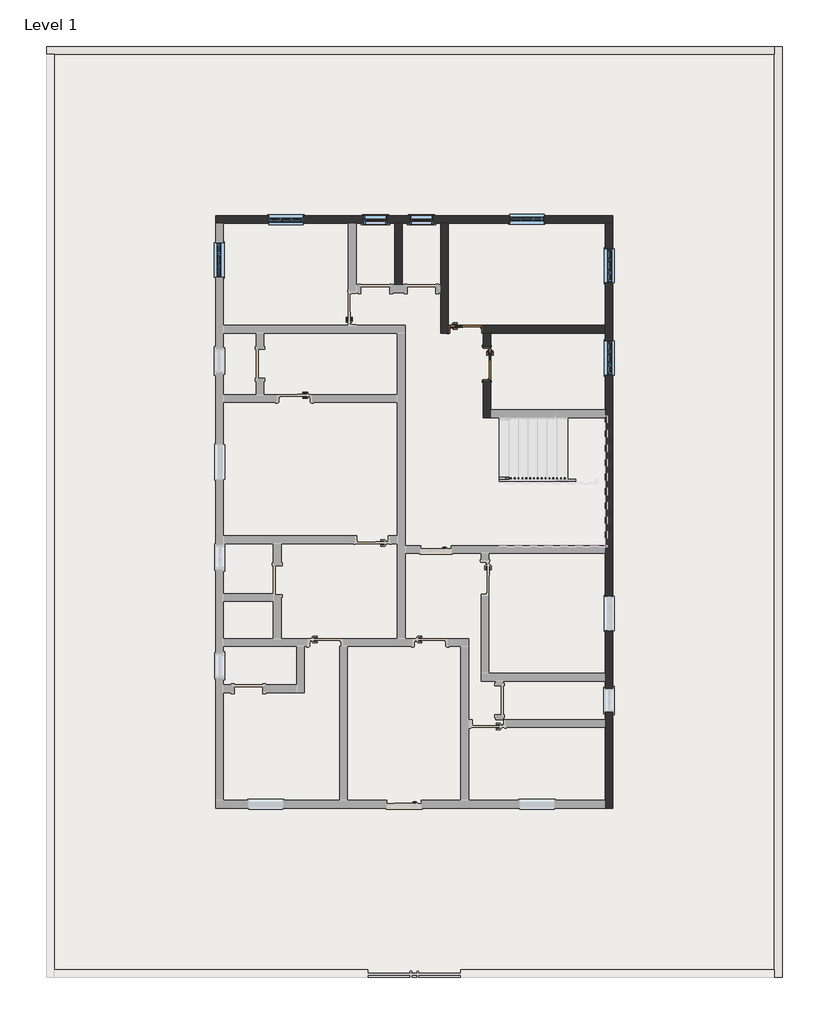
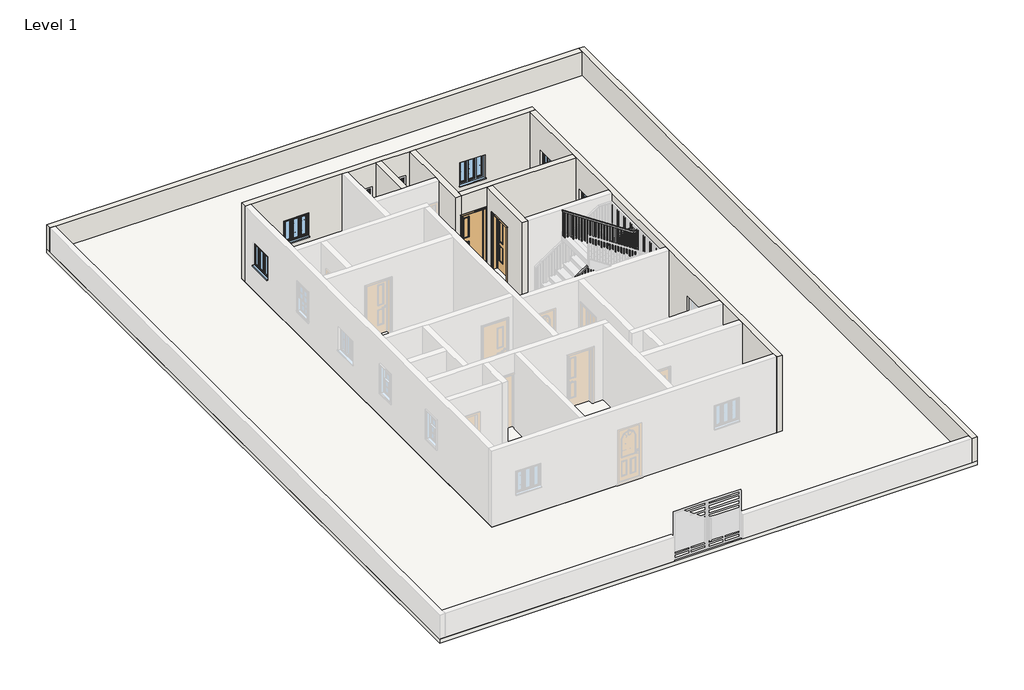
# One storey, part 2 of 3: 8 walls, 7 windows, 2 doors, 2 slabs, 1 railing.
"""IFC4 building model written with IfcOpenShell, lengths in millimetres."""

from ifc_helpers import new_model, si_unit, frame, origin, origin_with_axes, place, context, project, spatial, polyline, outline, extrude, faceted_brep, transform, mapped, element, save
from components import door_aa1d4bf3, window_679d2811, windows_tpl_w_glazing_bars_910x910mm_9d987a72

model = new_model("IFC4")

# Units and contexts
model_context = context("Model", 3, world=origin())
ifc_project = project(units=[si_unit("LENGTHUNIT", "METRE", prefix="MILLI")], contexts=[model_context])

# Site, building, storey
site = spatial("IfcSite", under=ifc_project)
building = spatial("IfcBuilding", under=site)
storey = spatial("IfcBuildingStorey", under=building, Name="Level 1", Elevation=0.0)

# Doors
placement = place(None, origin())
door_shape = door_aa1d4bf3(model_context)
element("IfcDoor", 1, ObjectType="Doors_IntSgl_3 : 7'-3\"", at=placement, inside=storey, context=model_context, shape_type="MappedRepresentation", body=[
    mapped(door_shape, transform((-7303.1711241, 14069.3344295, 0.0), x_axis=(1.0, 0.0, 0.0), y_axis=(0.0, 1.0, 0.0), z_axis=(0.0, 0.0, 1.0))),
])
element("IfcDoor", 2, ObjectType="Doors_IntSgl_3 : 7'-3\"", at=placement, inside=storey, context=model_context, shape_type="MappedRepresentation", body=[
    mapped(door_shape, transform((-6744.3711241, 13154.9344295, 0.0), x_axis=(0.0, -1.0, 0.0), y_axis=(1.0, 0.0, 0.0), z_axis=(0.0, 0.0, 1.0))),
])

# Railing
element("IfcRailing", 3, ObjectType="Handrail - Rectangular", at=placement, inside=storey, context=model_context, shape_type="SolidModel", body=[
    faceted_brep([(-6414.1711241, 10157.7344295, 1083.7333333), (-6414.1711241, 10157.7344295, 1022.6793317), (-6414.1711241, 10106.9344295, 1022.6793317), (-6414.1711241, 10106.9344295, 1083.7333333), (-4128.1711241, 10157.7344295, 2607.7333333), (-4112.7901217, 10157.7344295, 2556.9333333), (-4112.7901217, 10106.9344295, 2556.9333333), (-4128.1711241, 10106.9344295, 2607.7333333), (-3772.5711241, 10157.7344295, 2607.7333333), (-3772.5711241, 10157.7344295, 2556.9333333), (-3823.3711241, 10106.9344295, 2556.9333333), (-3823.3711241, 10106.9344295, 2607.7333333), (-3772.5711241, 9929.1344295, 2607.7333333), (-3772.5711241, 9929.1344295, 2556.9333333), (-3823.3711241, 9979.9344295, 2556.9333333), (-3823.3711241, 9979.9344295, 2607.7333333), (-3874.1711241, 9929.1344295, 2607.7333333), (-3889.5521265, 9929.1344295, 2556.9333333), (-3889.5521265, 9979.9344295, 2556.9333333), (-3874.1711241, 9979.9344295, 2607.7333333), (-6414.1711241, 9929.1344295, 4301.0666667), (-6414.1711241, 9979.9344295, 4301.0666667), (-6414.1711241, 9979.9344295, 4240.0126651), (-6414.1711241, 9929.1344295, 4240.0126651)], [[[0, 1, 2, 3]], [[1, 0, 4, 5]], [[2, 1, 5, 6]], [[3, 2, 6, 7]], [[0, 3, 7, 4]], [[5, 4, 8, 9]], [[6, 5, 9, 10]], [[7, 6, 10, 11]], [[4, 7, 11, 8]], [[9, 8, 12, 13]], [[10, 9, 13, 14]], [[11, 10, 14, 15]], [[8, 11, 15, 12]], [[13, 12, 16, 17]], [[14, 13, 17, 18]], [[15, 14, 18, 19]], [[12, 15, 19, 16]], [[20, 21, 22, 23]], [[17, 16, 20, 23]], [[18, 17, 23, 22]], [[19, 18, 22, 21]], [[16, 19, 21, 20]]]),
    extrude(outline(polyline([(4182.8626651, -6328.4461241), (4195.5626651, -6347.4961241), (3217.3333333, -6347.4961241), (3217.3333333, -6328.4461241), (4182.8626651, -6328.4461241)])), frame((0.0, 9945.0094295, 0.0), z_axis=(0.0, 1.0, 0.0), x_axis=(0.0, 0.0, 1.0)), (0.0, 0.0, 1.0), 19.05),
    extrude(outline(polyline([(4115.1293317, -6226.8461241), (4127.8293317, -6245.8961241), (3217.3333333, -6245.8961241), (3217.3333333, -6226.8461241), (4115.1293317, -6226.8461241)])), frame((0.0, 9945.0094295, 0.0), z_axis=(0.0, 1.0, 0.0), x_axis=(0.0, 0.0, 1.0)), (0.0, 0.0, 1.0), 19.05),
    extrude(outline(polyline([(4047.3959984, -6125.2461241), (4060.0959984, -6144.2961241), (3048.0, -6144.2961241), (3048.0, -6125.2461241), (4047.3959984, -6125.2461241)])), frame((0.0, 9945.0094295, 0.0), z_axis=(0.0, 1.0, 0.0), x_axis=(0.0, 0.0, 1.0)), (0.0, 0.0, 1.0), 19.05),
    extrude(outline(polyline([(3979.6626651, -6023.6461241), (3992.3626651, -6042.6961241), (3048.0, -6042.6961241), (3048.0, -6023.6461241), (3979.6626651, -6023.6461241)])), frame((0.0, 9945.0094295, 0.0), z_axis=(0.0, 1.0, 0.0), x_axis=(0.0, 0.0, 1.0)), (0.0, 0.0, 1.0), 19.05),
    extrude(outline(polyline([(3911.9293317, -5922.0461241), (3924.6293317, -5941.0961241), (3048.0, -5941.0961241), (3048.0, -5922.0461241), (3911.9293317, -5922.0461241)])), frame((0.0, 9945.0094295, 0.0), z_axis=(0.0, 1.0, 0.0), x_axis=(0.0, 0.0, 1.0)), (0.0, 0.0, 1.0), 19.05),
    extrude(outline(polyline([(3844.1959984, -5820.4461241), (3856.8959984, -5839.4961241), (2878.6666667, -5839.4961241), (2878.6666667, -5820.4461241), (3844.1959984, -5820.4461241)])), frame((0.0, 9945.0094295, 0.0), z_axis=(0.0, 1.0, 0.0), x_axis=(0.0, 0.0, 1.0)), (0.0, 0.0, 1.0), 19.05),
    extrude(outline(polyline([(3776.4626651, -5718.8461241), (3789.1626651, -5737.8961241), (2878.6666667, -5737.8961241), (2878.6666667, -5718.8461241), (3776.4626651, -5718.8461241)])), frame((0.0, 9945.0094295, 0.0), z_axis=(0.0, 1.0, 0.0), x_axis=(0.0, 0.0, 1.0)), (0.0, 0.0, 1.0), 19.05),
    extrude(outline(polyline([(3708.7293317, -5617.2461241), (3721.4293317, -5636.2961241), (2709.3333333, -5636.2961241), (2709.3333333, -5617.2461241), (3708.7293317, -5617.2461241)])), frame((0.0, 9945.0094295, 0.0), z_axis=(0.0, 1.0, 0.0), x_axis=(0.0, 0.0, 1.0)), (0.0, 0.0, 1.0), 19.05),
    extrude(outline(polyline([(3640.9959984, -5515.6461241), (3653.6959984, -5534.6961241), (2709.3333333, -5534.6961241), (2709.3333333, -5515.6461241), (3640.9959984, -5515.6461241)])), frame((0.0, 9945.0094295, 0.0), z_axis=(0.0, 1.0, 0.0), x_axis=(0.0, 0.0, 1.0)), (0.0, 0.0, 1.0), 19.05),
    extrude(outline(polyline([(3573.2626651, -5414.0461241), (3585.9626651, -5433.0961241), (2709.3333333, -5433.0961241), (2709.3333333, -5414.0461241), (3573.2626651, -5414.0461241)])), frame((0.0, 9945.0094295, 0.0), z_axis=(0.0, 1.0, 0.0), x_axis=(0.0, 0.0, 1.0)), (0.0, 0.0, 1.0), 19.05),
    extrude(outline(polyline([(3505.5293317, -5312.4461241), (3518.2293317, -5331.4961241), (2540.0, -5331.4961241), (2540.0, -5312.4461241), (3505.5293317, -5312.4461241)])), frame((0.0, 9945.0094295, 0.0), z_axis=(0.0, 1.0, 0.0), x_axis=(0.0, 0.0, 1.0)), (0.0, 0.0, 1.0), 19.05),
    extrude(outline(polyline([(3437.7959984, -5210.8461241), (3450.4959984, -5229.8961241), (2540.0, -5229.8961241), (2540.0, -5210.8461241), (3437.7959984, -5210.8461241)])), frame((0.0, 9945.0094295, 0.0), z_axis=(0.0, 1.0, 0.0), x_axis=(0.0, 0.0, 1.0)), (0.0, 0.0, 1.0), 19.05),
    extrude(outline(polyline([(3370.0626651, -5109.2461241), (3382.7626651, -5128.2961241), (2370.6666667, -5128.2961241), (2370.6666667, -5109.2461241), (3370.0626651, -5109.2461241)])), frame((0.0, 9945.0094295, 0.0), z_axis=(0.0, 1.0, 0.0), x_axis=(0.0, 0.0, 1.0)), (0.0, 0.0, 1.0), 19.05),
    extrude(outline(polyline([(3302.3293317, -5007.6461241), (3315.0293317, -5026.6961241), (2370.6666667, -5026.6961241), (2370.6666667, -5007.6461241), (3302.3293317, -5007.6461241)])), frame((0.0, 9945.0094295, 0.0), z_axis=(0.0, 1.0, 0.0), x_axis=(0.0, 0.0, 1.0)), (0.0, 0.0, 1.0), 19.05),
    extrude(outline(polyline([(3234.5959984, -4906.0461241), (3247.2959984, -4925.0961241), (2370.6666667, -4925.0961241), (2370.6666667, -4906.0461241), (3234.5959984, -4906.0461241)])), frame((0.0, 9945.0094295, 0.0), z_axis=(0.0, 1.0, 0.0), x_axis=(0.0, 0.0, 1.0)), (0.0, 0.0, 1.0), 19.05),
    extrude(outline(polyline([(3166.8626651, -4804.4461241), (3179.5626651, -4823.4961241), (2201.3333333, -4823.4961241), (2201.3333333, -4804.4461241), (3166.8626651, -4804.4461241)])), frame((0.0, 9945.0094295, 0.0), z_axis=(0.0, 1.0, 0.0), x_axis=(0.0, 0.0, 1.0)), (0.0, 0.0, 1.0), 19.05),
    extrude(outline(polyline([(3099.1293317, -4702.8461241), (3111.8293317, -4721.8961241), (2201.3333333, -4721.8961241), (2201.3333333, -4702.8461241), (3099.1293317, -4702.8461241)])), frame((0.0, 9945.0094295, 0.0), z_axis=(0.0, 1.0, 0.0), x_axis=(0.0, 0.0, 1.0)), (0.0, 0.0, 1.0), 19.05),
    extrude(outline(polyline([(3031.3959984, -4601.2461241), (3044.0959984, -4620.2961241), (2032.0, -4620.2961241), (2032.0, -4601.2461241), (3031.3959984, -4601.2461241)])), frame((0.0, 9945.0094295, 0.0), z_axis=(0.0, 1.0, 0.0), x_axis=(0.0, 0.0, 1.0)), (0.0, 0.0, 1.0), 19.05),
    extrude(outline(polyline([(2963.6626651, -4499.6461241), (2976.3626651, -4518.6961241), (2032.0, -4518.6961241), (2032.0, -4499.6461241), (2963.6626651, -4499.6461241)])), frame((0.0, 9945.0094295, 0.0), z_axis=(0.0, 1.0, 0.0), x_axis=(0.0, 0.0, 1.0)), (0.0, 0.0, 1.0), 19.05),
    extrude(outline(polyline([(2895.9293317, -4398.0461241), (2908.6293317, -4417.0961241), (2032.0, -4417.0961241), (2032.0, -4398.0461241), (2895.9293317, -4398.0461241)])), frame((0.0, 9945.0094295, 0.0), z_axis=(0.0, 1.0, 0.0), x_axis=(0.0, 0.0, 1.0)), (0.0, 0.0, 1.0), 19.05),
    extrude(outline(polyline([(2828.1959984, -4296.4461241), (2840.8959984, -4315.4961241), (1862.6666667, -4315.4961241), (1862.6666667, -4296.4461241), (2828.1959984, -4296.4461241)])), frame((0.0, 9945.0094295, 0.0), z_axis=(0.0, 1.0, 0.0), x_axis=(0.0, 0.0, 1.0)), (0.0, 0.0, 1.0), 19.05),
    extrude(outline(polyline([(2760.4626651, -4194.8461241), (2773.1626651, -4213.8961241), (1862.6666667, -4213.8961241), (1862.6666667, -4194.8461241), (2760.4626651, -4194.8461241)])), frame((0.0, 9945.0094295, 0.0), z_axis=(0.0, 1.0, 0.0), x_axis=(0.0, 0.0, 1.0)), (0.0, 0.0, 1.0), 19.05),
    extrude(outline(polyline([(2692.7293317, -4093.2461241), (2705.4293317, -4112.2961241), (1693.3333333, -4112.2961241), (1693.3333333, -4093.2461241), (2692.7293317, -4093.2461241)])), frame((0.0, 9945.0094295, 0.0), z_axis=(0.0, 1.0, 0.0), x_axis=(0.0, 0.0, 1.0)), (0.0, 0.0, 1.0), 19.05),
    extrude(outline(polyline([(2624.9959984, -3991.6461241), (2637.6959984, -4010.6961241), (1693.3333333, -4010.6961241), (1693.3333333, -3991.6461241), (2624.9959984, -3991.6461241)])), frame((0.0, 9945.0094295, 0.0), z_axis=(0.0, 1.0, 0.0), x_axis=(0.0, 0.0, 1.0)), (0.0, 0.0, 1.0), 19.05),
    extrude(outline(polyline([(2557.2626651, -3890.0461241), (2569.9626651, -3909.0961241), (1693.3333333, -3909.0961241), (1693.3333333, -3890.0461241), (2557.2626651, -3890.0461241)])), frame((0.0, 9945.0094295, 0.0), z_axis=(0.0, 1.0, 0.0), x_axis=(0.0, 0.0, 1.0)), (0.0, 0.0, 1.0), 19.05),
    extrude(outline(polyline([(-3807.4961241, 10040.2594295), (-3788.4461241, 10040.2594295), (-3788.4461241, 10021.2094295), (-3807.4961241, 10021.2094295), (-3807.4961241, 10040.2594295)])), frame((0.0, 0.0, 1693.3333333), z_axis=(0.0, 0.0, 1.0), x_axis=(1.0, 0.0, 0.0)), (0.0, 0.0, 1.0), 863.6),
    extrude(outline(polyline([(-3883.6961241, 10122.8094295), (-3883.6961241, 10141.8594295), (-3864.6461241, 10141.8594295), (-3864.6461241, 10122.8094295), (-3883.6961241, 10122.8094295)])), frame((0.0, 0.0, 1693.3333333), z_axis=(0.0, 0.0, 1.0), x_axis=(1.0, 0.0, 0.0)), (0.0, 0.0, 1.0), 863.6),
    extrude(outline(polyline([(-3985.2961241, 10122.8094295), (-3985.2961241, 10141.8594295), (-3966.2461241, 10141.8594295), (-3966.2461241, 10122.8094295), (-3985.2961241, 10122.8094295)])), frame((0.0, 0.0, 1693.3333333), z_axis=(0.0, 0.0, 1.0), x_axis=(1.0, 0.0, 0.0)), (0.0, 0.0, 1.0), 863.6),
    extrude(outline(polyline([(-4086.8961241, 10122.8094295), (-4086.8961241, 10141.8594295), (-4067.8461241, 10141.8594295), (-4067.8461241, 10122.8094295), (-4086.8961241, 10122.8094295)])), frame((0.0, 0.0, 1693.3333333), z_axis=(0.0, 0.0, 1.0), x_axis=(1.0, 0.0, 0.0)), (0.0, 0.0, 1.0), 863.6),
    extrude(outline(polyline([(2519.1626651, -4169.4461241), (2506.4626651, -4188.4961241), (1524.0, -4188.4961241), (1524.0, -4169.4461241), (2519.1626651, -4169.4461241)])), frame((0.0, 10122.8094295, 0.0), z_axis=(0.0, 1.0, 0.0), x_axis=(0.0, 0.0, 1.0)), (0.0, 0.0, 1.0), 19.05),
    extrude(outline(polyline([(2451.4293317, -4271.0461241), (2438.7293317, -4290.0961241), (1524.0, -4290.0961241), (1524.0, -4271.0461241), (2451.4293317, -4271.0461241)])), frame((0.0, 10122.8094295, 0.0), z_axis=(0.0, 1.0, 0.0), x_axis=(0.0, 0.0, 1.0)), (0.0, 0.0, 1.0), 19.05),
    extrude(outline(polyline([(2383.6959984, -4372.6461241), (2370.9959984, -4391.6961241), (1524.0, -4391.6961241), (1524.0, -4372.6461241), (2383.6959984, -4372.6461241)])), frame((0.0, 10122.8094295, 0.0), z_axis=(0.0, 1.0, 0.0), x_axis=(0.0, 0.0, 1.0)), (0.0, 0.0, 1.0), 19.05),
    extrude(outline(polyline([(2315.9626651, -4474.2461241), (2303.2626651, -4493.2961241), (1354.6666667, -4493.2961241), (1354.6666667, -4474.2461241), (2315.9626651, -4474.2461241)])), frame((0.0, 10122.8094295, 0.0), z_axis=(0.0, 1.0, 0.0), x_axis=(0.0, 0.0, 1.0)), (0.0, 0.0, 1.0), 19.05),
    extrude(outline(polyline([(2248.2293317, -4575.8461241), (2235.5293317, -4594.8961241), (1354.6666667, -4594.8961241), (1354.6666667, -4575.8461241), (2248.2293317, -4575.8461241)])), frame((0.0, 10122.8094295, 0.0), z_axis=(0.0, 1.0, 0.0), x_axis=(0.0, 0.0, 1.0)), (0.0, 0.0, 1.0), 19.05),
    extrude(outline(polyline([(2180.4959984, -4677.4461241), (2167.7959984, -4696.4961241), (1185.3333333, -4696.4961241), (1185.3333333, -4677.4461241), (2180.4959984, -4677.4461241)])), frame((0.0, 10122.8094295, 0.0), z_axis=(0.0, 1.0, 0.0), x_axis=(0.0, 0.0, 1.0)), (0.0, 0.0, 1.0), 19.05),
    extrude(outline(polyline([(2112.7626651, -4779.0461241), (2100.0626651, -4798.0961241), (1185.3333333, -4798.0961241), (1185.3333333, -4779.0461241), (2112.7626651, -4779.0461241)])), frame((0.0, 10122.8094295, 0.0), z_axis=(0.0, 1.0, 0.0), x_axis=(0.0, 0.0, 1.0)), (0.0, 0.0, 1.0), 19.05),
    extrude(outline(polyline([(2045.0293317, -4880.6461241), (2032.3293317, -4899.6961241), (1185.3333333, -4899.6961241), (1185.3333333, -4880.6461241), (2045.0293317, -4880.6461241)])), frame((0.0, 10122.8094295, 0.0), z_axis=(0.0, 1.0, 0.0), x_axis=(0.0, 0.0, 1.0)), (0.0, 0.0, 1.0), 19.05),
    extrude(outline(polyline([(1977.2959984, -4982.2461241), (1964.5959984, -5001.2961241), (1016.0, -5001.2961241), (1016.0, -4982.2461241), (1977.2959984, -4982.2461241)])), frame((0.0, 10122.8094295, 0.0), z_axis=(0.0, 1.0, 0.0), x_axis=(0.0, 0.0, 1.0)), (0.0, 0.0, 1.0), 19.05),
    extrude(outline(polyline([(1909.5626651, -5083.8461241), (1896.8626651, -5102.8961241), (1016.0, -5102.8961241), (1016.0, -5083.8461241), (1909.5626651, -5083.8461241)])), frame((0.0, 10122.8094295, 0.0), z_axis=(0.0, 1.0, 0.0), x_axis=(0.0, 0.0, 1.0)), (0.0, 0.0, 1.0), 19.05),
    extrude(outline(polyline([(1841.8293317, -5185.4461241), (1829.1293317, -5204.4961241), (846.6666667, -5204.4961241), (846.6666667, -5185.4461241), (1841.8293317, -5185.4461241)])), frame((0.0, 10122.8094295, 0.0), z_axis=(0.0, 1.0, 0.0), x_axis=(0.0, 0.0, 1.0)), (0.0, 0.0, 1.0), 19.05),
    extrude(outline(polyline([(1774.0959984, -5287.0461241), (1761.3959984, -5306.0961241), (846.6666667, -5306.0961241), (846.6666667, -5287.0461241), (1774.0959984, -5287.0461241)])), frame((0.0, 10122.8094295, 0.0), z_axis=(0.0, 1.0, 0.0), x_axis=(0.0, 0.0, 1.0)), (0.0, 0.0, 1.0), 19.05),
    extrude(outline(polyline([(1706.3626651, -5388.6461241), (1693.6626651, -5407.6961241), (846.6666667, -5407.6961241), (846.6666667, -5388.6461241), (1706.3626651, -5388.6461241)])), frame((0.0, 10122.8094295, 0.0), z_axis=(0.0, 1.0, 0.0), x_axis=(0.0, 0.0, 1.0)), (0.0, 0.0, 1.0), 19.05),
    extrude(outline(polyline([(1638.6293317, -5490.2461241), (1625.9293317, -5509.2961241), (677.3333333, -5509.2961241), (677.3333333, -5490.2461241), (1638.6293317, -5490.2461241)])), frame((0.0, 10122.8094295, 0.0), z_axis=(0.0, 1.0, 0.0), x_axis=(0.0, 0.0, 1.0)), (0.0, 0.0, 1.0), 19.05),
    extrude(outline(polyline([(1570.8959984, -5591.8461241), (1558.1959984, -5610.8961241), (677.3333333, -5610.8961241), (677.3333333, -5591.8461241), (1570.8959984, -5591.8461241)])), frame((0.0, 10122.8094295, 0.0), z_axis=(0.0, 1.0, 0.0), x_axis=(0.0, 0.0, 1.0)), (0.0, 0.0, 1.0), 19.05),
    extrude(outline(polyline([(1503.1626651, -5693.4461241), (1490.4626651, -5712.4961241), (508.0, -5712.4961241), (508.0, -5693.4461241), (1503.1626651, -5693.4461241)])), frame((0.0, 10122.8094295, 0.0), z_axis=(0.0, 1.0, 0.0), x_axis=(0.0, 0.0, 1.0)), (0.0, 0.0, 1.0), 19.05),
    extrude(outline(polyline([(1435.4293317, -5795.0461241), (1422.7293317, -5814.0961241), (508.0, -5814.0961241), (508.0, -5795.0461241), (1435.4293317, -5795.0461241)])), frame((0.0, 10122.8094295, 0.0), z_axis=(0.0, 1.0, 0.0), x_axis=(0.0, 0.0, 1.0)), (0.0, 0.0, 1.0), 19.05),
    extrude(outline(polyline([(1367.6959984, -5896.6461241), (1354.9959984, -5915.6961241), (508.0, -5915.6961241), (508.0, -5896.6461241), (1367.6959984, -5896.6461241)])), frame((0.0, 10122.8094295, 0.0), z_axis=(0.0, 1.0, 0.0), x_axis=(0.0, 0.0, 1.0)), (0.0, 0.0, 1.0), 19.05),
    extrude(outline(polyline([(1299.9626651, -5998.2461241), (1287.2626651, -6017.2961241), (338.6666667, -6017.2961241), (338.6666667, -5998.2461241), (1299.9626651, -5998.2461241)])), frame((0.0, 10122.8094295, 0.0), z_axis=(0.0, 1.0, 0.0), x_axis=(0.0, 0.0, 1.0)), (0.0, 0.0, 1.0), 19.05),
    extrude(outline(polyline([(1232.2293317, -6099.8461241), (1219.5293317, -6118.8961241), (338.6666667, -6118.8961241), (338.6666667, -6099.8461241), (1232.2293317, -6099.8461241)])), frame((0.0, 10122.8094295, 0.0), z_axis=(0.0, 1.0, 0.0), x_axis=(0.0, 0.0, 1.0)), (0.0, 0.0, 1.0), 19.05),
    extrude(outline(polyline([(1164.4959984, -6201.4461241), (1151.7959984, -6220.4961241), (169.3333333, -6220.4961241), (169.3333333, -6201.4461241), (1164.4959984, -6201.4461241)])), frame((0.0, 10122.8094295, 0.0), z_axis=(0.0, 1.0, 0.0), x_axis=(0.0, 0.0, 1.0)), (0.0, 0.0, 1.0), 19.05),
    extrude(outline(polyline([(1096.7626651, -6303.0461241), (1084.0626651, -6322.0961241), (169.3333333, -6322.0961241), (169.3333333, -6303.0461241), (1096.7626651, -6303.0461241)])), frame((0.0, 10122.8094295, 0.0), z_axis=(0.0, 1.0, 0.0), x_axis=(0.0, 0.0, 1.0)), (0.0, 0.0, 1.0), 19.05),
    extrude(outline(polyline([(-3807.4961241, 9964.0594295), (-3788.4461241, 9964.0594295), (-3788.4461241, 9945.0094295), (-3807.4961241, 9945.0094295), (-3807.4961241, 9964.0594295)])), frame((0.0, 0.0, 1693.3333333), z_axis=(0.0, 0.0, 1.0), x_axis=(1.0, 0.0, 0.0)), (0.0, 0.0, 1.0), 863.6),
    extrude(outline(polyline([(-3807.4961241, 10122.8094295), (-3807.4961241, 10141.8594295), (-3788.4461241, 10141.8594295), (-3788.4461241, 10122.8094295), (-3807.4961241, 10122.8094295)])), frame((0.0, 0.0, 1693.3333333), z_axis=(0.0, 0.0, 1.0), x_axis=(1.0, 0.0, 0.0)), (0.0, 0.0, 1.0), 863.6),
    extrude(outline(polyline([(4227.3126651, -6395.1211241), (4240.0126651, -6414.1711241), (3217.3333333, -6414.1711241), (3217.3333333, -6395.1211241), (4227.3126651, -6395.1211241)])), frame((0.0, 9945.0094295, 0.0), z_axis=(0.0, 1.0, 0.0), x_axis=(0.0, 0.0, 1.0)), (0.0, 0.0, 1.0), 19.05),
    extrude(outline(polyline([(1035.3793317, -6395.1211241), (1022.6793317, -6414.1711241), (169.3333333, -6414.1711241), (169.3333333, -6395.1211241), (1035.3793317, -6395.1211241)])), frame((0.0, 10122.8094295, 0.0), z_axis=(0.0, 1.0, 0.0), x_axis=(0.0, 0.0, 1.0)), (0.0, 0.0, 1.0), 19.05),
])

# Slabs
element("IfcSlab", 4, ObjectType="Generic - 12\"", at=placement, inside=storey, context=model_context, shape_type="SweptSolid", body=[
    extrude(outline(polyline([(1053.4288759, 21536.9344295), (1053.4288759, -3050.2655705), (-18377.5711241, -3050.2655705), (-18377.5711241, 21536.9344295), (1053.4288759, 21536.9344295)])), frame((0.0, 0.0, -152.4), z_axis=(0.0, 0.0, 1.0), x_axis=(1.0, 0.0, 0.0)), (0.0, 0.0, 1.0), 152.4),
])
element("IfcSlab", 5, ObjectType="Generic - 12\" 2", at=placement, inside=storey, context=model_context, shape_type="SweptSolid", body=[
    extrude(outline(polyline([(-3416.9711241, 17066.5344295), (-3416.9711241, 1420.1344295), (-13907.1711241, 1420.1344295), (-13907.1711241, 17066.5344295), (-3416.9711241, 17066.5344295)])), frame((0.0, 0.0, -152.4), z_axis=(0.0, 0.0, 1.0), x_axis=(1.0, 0.0, 0.0)), (0.0, 0.0, 1.0), 152.4),
])

# Walls
element("IfcWall", 6, ObjectType="Generic -4.5\" p", at=placement, inside=storey, context=model_context, shape_type="SweptSolid", body=[
    extrude(outline(polyline([(-9182.7711241, 15237.7344295), (-9182.7711241, 16863.3344295), (-8979.5711241, 16863.3344295), (-8979.5711241, 15237.7344295), (-9182.7711241, 15237.7344295)])), origin_with_axes(), (0.0, 0.0, 1.0), 2895.6),
])
element("IfcWall", 7, ObjectType="Generic -4.5\" p", at=placement, inside=storey, context=model_context, shape_type="Brep", body=[
    faceted_brep([(-7963.5711241, 16863.3344295, 0.0), (-7963.5711241, 15237.7344295, 0.0), (-7963.5711241, 15034.5344295, 0.0), (-7963.5711241, 13967.7344295, 0.0), (-7963.5711241, 13967.7344295, 2895.6), (-7963.5711241, 15034.5344295, 2895.6), (-7963.5711241, 15237.7344295, 2895.6), (-7963.5711241, 16863.3344295, 2895.6), (-7760.3711241, 16863.3344295, 0.0), (-7760.3711241, 16863.3344295, 2895.6), (-7760.3711241, 14170.9344295, 2895.6), (-7760.3711241, 13967.7344295, 2895.6), (-7760.3711241, 13967.7344295, 2133.6), (-7760.3711241, 13967.7344295, 0.0)], [[[0, 1, 2, 3, 4, 5, 6, 7]], [[8, 9, 10, 11, 12, 13]], [[3, 2, 1, 0, 8, 13]], [[0, 7, 9, 8]], [[4, 3, 13, 12, 11]], [[7, 6, 5, 4, 11, 10, 9]]]),
])
element("IfcWall", 8, ObjectType="Generic -4.5\" p", at=placement, inside=storey, context=model_context, shape_type="Brep", body=[
    faceted_brep([(-3620.1711241, 14170.9344295, 2895.6), (-3620.1711241, 14170.9344295, 0.0), (-6845.9711241, 14170.9344295, 0.0), (-6845.9711241, 14170.9344295, 2133.6), (-7760.3711241, 14170.9344295, 2133.6), (-7760.3711241, 14170.9344295, 2895.6), (-3620.1711241, 13967.7344295, 0.0), (-3620.1711241, 13967.7344295, 2895.6), (-6642.7711241, 13967.7344295, 2895.6), (-6845.9711241, 13967.7344295, 2895.6), (-7760.3711241, 13967.7344295, 2895.6), (-7760.3711241, 13967.7344295, 2133.6), (-6845.9711241, 13967.7344295, 2133.6), (-6845.9711241, 13967.7344295, 0.0), (-6642.7711241, 13967.7344295, 0.0)], [[[0, 1, 2, 3, 4, 5]], [[6, 7, 8, 9, 10, 11, 12, 13, 14]], [[1, 6, 14, 13, 2]], [[10, 5, 4, 11]], [[1, 0, 7, 6]], [[12, 3, 2, 13]], [[3, 12, 11, 4]], [[0, 5, 10, 9, 8, 7]]]),
])
element("IfcWall", 9, ObjectType="Generic -4.5\" p", at=placement, inside=storey, context=model_context, shape_type="Brep", body=[
    faceted_brep([(-6845.9711241, 13967.7344295, 2895.6), (-6845.9711241, 13967.7344295, 2133.6), (-6845.9711241, 13967.7344295, 0.0), (-6845.9711241, 13612.1344295, 0.0), (-6845.9711241, 13612.1344295, 2133.6), (-6845.9711241, 12697.7344295, 2133.6), (-6845.9711241, 12697.7344295, 0.0), (-6845.9711241, 11732.5344295, 0.0), (-6845.9711241, 11732.5344295, 2895.6), (-6642.7711241, 13967.7344295, 0.0), (-6642.7711241, 13967.7344295, 2895.6), (-6642.7711241, 11935.7344295, 2895.6), (-6642.7711241, 11732.5344295, 2895.6), (-6642.7711241, 11732.5344295, 0.0), (-6642.7711241, 11935.7344295, 0.0), (-6642.7711241, 12697.7344295, 0.0), (-6642.7711241, 12697.7344295, 2133.6), (-6642.7711241, 13612.1344295, 2133.6), (-6642.7711241, 13612.1344295, 0.0)], [[[0, 1, 2, 3, 4, 5, 6, 7, 8]], [[9, 10, 11, 12, 13, 14, 15, 16, 17, 18]], [[2, 9, 18, 3]], [[13, 7, 6, 15, 14]], [[2, 1, 0, 10, 9]], [[8, 7, 13, 12]], [[5, 16, 15, 6]], [[16, 5, 4, 17]], [[17, 4, 3, 18]], [[0, 8, 12, 11, 10]]]),
])
element("IfcWall", 10, ObjectType="Generic -4.5\" p", at=placement, inside=storey, context=model_context, shape_type="Brep", body=[
    faceted_brep([(-18377.5711241, 21333.7344295, 0.0), (-18174.3711241, 21333.7344295, 0.0), (850.2288759, 21333.7344295, 0.0), (850.2288759, 21333.7344295, 914.4), (-18174.3711241, 21333.7344295, 914.4), (-18377.5711241, 21333.7344295, 914.4), (-18377.5711241, 21536.9344295, 0.0), (-18377.5711241, 21536.9344295, 914.4), (850.2288759, 21536.9344295, 914.4), (850.2288759, 21536.9344295, 0.0)], [[[0, 1, 2, 3, 4, 5]], [[6, 7, 8, 9]], [[2, 1, 0, 6, 9]], [[5, 4, 3, 8, 7]], [[0, 5, 7, 6]], [[3, 2, 9, 8]]]),
])
element("IfcWall", 11, ObjectType="Generic -4.5\" p", at=placement, inside=storey, context=model_context, shape_type="Brep", body=[
    faceted_brep([(850.2288759, 21536.9344295, 0.0), (850.2288759, 21333.7344295, 0.0), (850.2288759, -2847.0655705, 0.0), (850.2288759, -3050.2655705, 0.0), (850.2288759, -3050.2655705, 914.4), (850.2288759, -2847.0655705, 914.4), (850.2288759, 21333.7344295, 914.4), (850.2288759, 21536.9344295, 914.4), (1053.4288759, 21536.9344295, 0.0), (1053.4288759, 21536.9344295, 914.4), (1053.4288759, -3050.2655705, 914.4), (1053.4288759, -3050.2655705, 0.0)], [[[0, 1, 2, 3, 4, 5, 6, 7]], [[8, 9, 10, 11]], [[3, 2, 1, 0, 8, 11]], [[7, 6, 5, 4, 10, 9]], [[0, 7, 9, 8]], [[4, 3, 11, 10]]]),
])
element("IfcWall", 12, ObjectType="Generic -9\" w", at=placement, inside=storey, context=model_context, shape_type="Brep", body=[
    faceted_brep([(-13907.1711241, 16863.3344295, 0.0), (-13703.9711241, 16863.3344295, 0.0), (-10401.9711241, 16863.3344295, 0.0), (-10198.7711241, 16863.3344295, 0.0), (-9182.7711241, 16863.3344295, 0.0), (-8979.5711241, 16863.3344295, 0.0), (-7963.5711241, 16863.3344295, 0.0), (-7760.3711241, 16863.3344295, 0.0), (-3620.1711241, 16863.3344295, 0.0), (-3416.9711241, 16863.3344295, 0.0), (-3416.9711241, 16863.3344295, 2895.6), (-3620.1711241, 16863.3344295, 2895.6), (-7760.3711241, 16863.3344295, 2895.6), (-7963.5711241, 16863.3344295, 2895.6), (-8979.5711241, 16863.3344295, 2895.6), (-9182.7711241, 16863.3344295, 2895.6), (-10198.7711241, 16863.3344295, 2895.6), (-10401.9711241, 16863.3344295, 2895.6), (-13703.9711241, 16863.3344295, 2895.6), (-13907.1711241, 16863.3344295, 2895.6), (-11597.9711241, 16863.3344295, 1824.4), (-11597.9711241, 16863.3344295, 914.4), (-12507.9711241, 16863.3344295, 914.4), (-12507.9711241, 16863.3344295, 1824.4), (-6145.2711241, 16863.3344295, 1824.4), (-5235.2711241, 16863.3344295, 1824.4), (-5235.2711241, 16863.3344295, 914.4), (-6145.2711241, 16863.3344295, 914.4), (-9385.9711241, 16863.3344295, 1981.2), (-9385.9711241, 16863.3344295, 914.4), (-9995.5711241, 16863.3344295, 914.4), (-9995.5711241, 16863.3344295, 1981.2), (-8166.7711241, 16863.3344295, 1981.2), (-8166.7711241, 16863.3344295, 914.4), (-8776.3711241, 16863.3344295, 914.4), (-8776.3711241, 16863.3344295, 1981.2), (-13907.1711241, 17066.5344295, 0.0), (-13907.1711241, 17066.5344295, 2895.6), (-3416.9711241, 17066.5344295, 2895.6), (-3416.9711241, 17066.5344295, 0.0), (-11597.9711241, 17066.5344295, 1824.4), (-12507.9711241, 17066.5344295, 1824.4), (-12507.9711241, 17066.5344295, 914.4), (-11597.9711241, 17066.5344295, 914.4), (-6145.2711241, 17066.5344295, 1824.4), (-6145.2711241, 17066.5344295, 914.4), (-5235.2711241, 17066.5344295, 914.4), (-5235.2711241, 17066.5344295, 1824.4), (-9385.9711241, 17066.5344295, 1981.2), (-9995.5711241, 17066.5344295, 1981.2), (-9995.5711241, 17066.5344295, 914.4), (-9385.9711241, 17066.5344295, 914.4), (-8166.7711241, 17066.5344295, 1981.2), (-8776.3711241, 17066.5344295, 1981.2), (-8776.3711241, 17066.5344295, 914.4), (-8166.7711241, 17066.5344295, 914.4)], [[[0, 1, 2, 3, 4, 5, 6, 7, 8, 9, 10, 11, 12, 13, 14, 15, 16, 17, 18, 19], [20, 21, 22, 23], [24, 25, 26, 27], [28, 29, 30, 31], [32, 33, 34, 35]], [[36, 37, 38, 39], [40, 41, 42, 43], [44, 45, 46, 47], [48, 49, 50, 51], [52, 53, 54, 55]], [[9, 8, 7, 6, 5, 4, 3, 2, 1, 0, 36, 39]], [[10, 9, 39, 38]], [[0, 19, 37, 36]], [[21, 20, 40, 43]], [[22, 21, 43, 42]], [[23, 22, 42, 41]], [[20, 23, 41, 40]], [[45, 44, 24, 27]], [[46, 45, 27, 26]], [[47, 46, 26, 25]], [[44, 47, 25, 24]], [[29, 28, 48, 51]], [[30, 29, 51, 50]], [[31, 30, 50, 49]], [[28, 31, 49, 48]], [[33, 32, 52, 55]], [[34, 33, 55, 54]], [[35, 34, 54, 53]], [[32, 35, 53, 52]], [[19, 18, 17, 16, 15, 14, 13, 12, 11, 10, 38, 37]]]),
])
element("IfcWall", 13, ObjectType="Generic -9\" w", at=placement, inside=storey, context=model_context, shape_type="Brep", body=[
    faceted_brep([(-3620.1711241, 16863.3344295, 0.0), (-3620.1711241, 14170.9344295, 0.0), (-3620.1711241, 13967.7344295, 0.0), (-3620.1711241, 11935.7344295, 0.0), (-3620.1711241, 11732.5344295, 0.0), (-3620.1711241, 8354.3344295, 0.0), (-3620.1711241, 8151.1344295, 0.0), (-3620.1711241, 4976.1344295, 0.0), (-3620.1711241, 4772.9344295, 0.0), (-3620.1711241, 3756.9344295, 0.0), (-3620.1711241, 3553.7344295, 0.0), (-3620.1711241, 1623.3344295, 0.0), (-3620.1711241, 1420.1344295, 0.0), (-3620.1711241, 1420.1344295, 2895.6), (-3620.1711241, 1623.3344295, 2895.6), (-3620.1711241, 3553.7344295, 2895.6), (-3620.1711241, 3756.9344295, 2895.6), (-3620.1711241, 4772.9344295, 2895.6), (-3620.1711241, 4976.1344295, 2895.6), (-3620.1711241, 8151.1344295, 2895.6), (-3620.1711241, 8354.3344295, 2895.6), (-3620.1711241, 11732.5344295, 2895.6), (-3620.1711241, 11935.7344295, 2895.6), (-3620.1711241, 13967.7344295, 2895.6), (-3620.1711241, 14170.9344295, 2895.6), (-3620.1711241, 16863.3344295, 2895.6), (-3620.1711241, 16200.7344295, 1824.4), (-3620.1711241, 15290.7344295, 1824.4), (-3620.1711241, 15290.7344295, 914.4), (-3620.1711241, 16200.7344295, 914.4), (-3620.1711241, 13762.3344295, 1824.4), (-3620.1711241, 12852.3344295, 1824.4), (-3620.1711241, 12852.3344295, 914.4), (-3620.1711241, 13762.3344295, 914.4), (-3620.1711241, 7018.6344295, 1824.4), (-3620.1711241, 6108.6344295, 1824.4), (-3620.1711241, 6108.6344295, 914.4), (-3620.1711241, 7018.6344295, 914.4), (-3620.1711241, 4569.7344295, 1981.2), (-3620.1711241, 3960.1344295, 1981.2), (-3620.1711241, 3960.1344295, 914.4), (-3620.1711241, 4569.7344295, 914.4), (-3416.9711241, 16863.3344295, 0.0), (-3416.9711241, 16863.3344295, 2895.6), (-3416.9711241, 1420.1344295, 2895.6), (-3416.9711241, 1420.1344295, 0.0), (-3416.9711241, 16200.7344295, 1824.4), (-3416.9711241, 16200.7344295, 914.4), (-3416.9711241, 15290.7344295, 914.4), (-3416.9711241, 15290.7344295, 1824.4), (-3416.9711241, 13762.3344295, 1824.4), (-3416.9711241, 13762.3344295, 914.4), (-3416.9711241, 12852.3344295, 914.4), (-3416.9711241, 12852.3344295, 1824.4), (-3416.9711241, 7018.6344295, 1824.4), (-3416.9711241, 7018.6344295, 914.4), (-3416.9711241, 6108.6344295, 914.4), (-3416.9711241, 6108.6344295, 1824.4), (-3416.9711241, 4569.7344295, 1981.2), (-3416.9711241, 4569.7344295, 914.4), (-3416.9711241, 3960.1344295, 914.4), (-3416.9711241, 3960.1344295, 1981.2)], [[[0, 1, 2, 3, 4, 5, 6, 7, 8, 9, 10, 11, 12, 13, 14, 15, 16, 17, 18, 19, 20, 21, 22, 23, 24, 25], [26, 27, 28, 29], [30, 31, 32, 33], [34, 35, 36, 37], [38, 39, 40, 41]], [[42, 43, 44, 45], [46, 47, 48, 49], [50, 51, 52, 53], [54, 55, 56, 57], [58, 59, 60, 61]], [[12, 11, 10, 9, 8, 7, 6, 5, 4, 3, 2, 1, 0, 42, 45]], [[0, 25, 43, 42]], [[13, 12, 45, 44]], [[47, 46, 26, 29]], [[48, 47, 29, 28]], [[49, 48, 28, 27]], [[46, 49, 27, 26]], [[51, 50, 30, 33]], [[52, 51, 33, 32]], [[53, 52, 32, 31]], [[50, 53, 31, 30]], [[55, 54, 34, 37]], [[56, 55, 37, 36]], [[57, 56, 36, 35]], [[54, 57, 35, 34]], [[59, 58, 38, 41]], [[60, 59, 41, 40]], [[61, 60, 40, 39]], [[58, 61, 39, 38]], [[25, 24, 23, 22, 21, 20, 19, 18, 17, 16, 15, 14, 13, 44, 43]]]),
])

# Windows
window_shape = window_679d2811(model_context)
element("IfcWindow", 14, ObjectType="Window-Double-Hung : 24\" x 42\"", at=placement, inside=storey, context=model_context, shape_type="MappedRepresentation", body=[
    mapped(window_shape, transform((-9690.7711241, 16964.9344295, 0.0), x_axis=(-1.0, 0.0, 0.0), y_axis=(0.0, -1.0, 0.0), z_axis=(0.0, 0.0, 1.0))),
])
element("IfcWindow", 15, ObjectType="Window-Double-Hung : 24\" x 42\"", at=placement, inside=storey, context=model_context, shape_type="MappedRepresentation", body=[
    mapped(window_shape, transform((-8471.5711241, 16964.9344295, 0.0), x_axis=(-1.0, 0.0, 0.0), y_axis=(0.0, -1.0, 0.0), z_axis=(0.0, 0.0, 1.0))),
])
windows_tpl_w_glazing_bars_910x910mm_shape = windows_tpl_w_glazing_bars_910x910mm_9d987a72(model_context)
element("IfcWindow", 16, ObjectType="Windows_Tpl_w-Glazing_Bars : 910x910mm", at=placement, inside=storey, context=model_context, shape_type="MappedRepresentation", body=[
    mapped(windows_tpl_w_glazing_bars_910x910mm_shape, transform((-12289.6377907, 16973.3909974, -285.6), x_axis=(-1.0, 0.0, 0.0), y_axis=(0.0, -1.0, 0.0), z_axis=(0.0, 0.0, 1.0))),
])
element("IfcWindow", 17, ObjectType="Windows_Tpl_w-Glazing_Bars : 910x910mm", at=placement, inside=storey, context=model_context, shape_type="MappedRepresentation", body=[
    mapped(windows_tpl_w_glazing_bars_910x910mm_shape, transform((-5453.6044574, 16956.4778617, -285.6), x_axis=(1.0, 0.0, 0.0), y_axis=(0.0, 1.0, 0.0), z_axis=(0.0, 0.0, 1.0))),
])
element("IfcWindow", 18, ObjectType="Windows_Tpl_w-Glazing_Bars : 910x910mm", at=placement, inside=storey, context=model_context, shape_type="MappedRepresentation", body=[
    mapped(windows_tpl_w_glazing_bars_910x910mm_shape, transform((-3527.0276919, 15509.0677629, -285.6), x_axis=(0.0, -1.0, 0.0), y_axis=(1.0, 0.0, 0.0), z_axis=(0.0, 0.0, 1.0))),
])
element("IfcWindow", 19, ObjectType="Windows_Tpl_w-Glazing_Bars : 910x910mm", at=placement, inside=storey, context=model_context, shape_type="MappedRepresentation", body=[
    mapped(windows_tpl_w_glazing_bars_910x910mm_shape, transform((-13797.1145562, 16134.8010962, -285.6), x_axis=(0.0, 1.0, 0.0), y_axis=(-1.0, 0.0, 0.0), z_axis=(0.0, 0.0, 1.0))),
])
element("IfcWindow", 20, ObjectType="Windows_Tpl_w-Glazing_Bars : 910x910mm", at=placement, inside=storey, context=model_context, shape_type="MappedRepresentation", body=[
    mapped(windows_tpl_w_glazing_bars_910x910mm_shape, transform((-3527.0276919, 13070.6677629, -285.6), x_axis=(0.0, -1.0, 0.0), y_axis=(1.0, 0.0, 0.0), z_axis=(0.0, 0.0, 1.0))),
])

save(model, "model.ifc")

# Revit data of these elements
# Type "Doors_IntSgl_3 : 7'-3\""
#   Type Mark = "14"
#   Type Comments = "Internal Single"
#   Operation = "SingleSwingRight"
#   Construction Type Id = "SGL"
#   Manufacturer = "Revit"
#   Keynote = "L20"
#   Description = "Internal Single Door"
#   Analytic Construction = "Large single-glazed windows"
#   Visual Light Transmittance = 0.9
#   VisionPanel Width = 0' - 7.87402"
#   UnderCut = 0' - 0.31496"
#   Tolerance = 0' - 0.07874"
#   Structural Tolerance = 0' - 0.31496"
#   StopDepth = 0' - 1.25984"
#   Stop Thickness = 0' - 0.74803"
#   Stile Top of Lock Rail = 3' - 7.30709"
#   Stile Top Rail = 0' - 8.85827"
#   Stile Shutting = 0' - 4.92126"
#   Stile Lock Rail = 0' - 6.88976"
#   Stile Bottom Rail = 1' - 1.77953"
#   Solar Heat Gain Coefficient = 0.86
#   Rough Width = 3' - 0"
#   Rough Height = 7' - 0"
#   Heat Transfer Coefficient (U) = 0.979472 BTU/(h·ft²·°F)
#   Handle Z Distance = 3' - 3.37008"
#   Handle X Distance = 0' - 2.95276"
#   Frame Thickness = 0' - 1.25984"
#   Door Panel Width = 2' - 8.69291"
#   Door Panel Thickness = 0' - 1.49606"
#   Door Panel Offset = 0' - 0"
#   Height = 7' - 0"
#   Width = 3' - 0"
#   Door Panel Height = 6' - 10.0315"
#   Architrave Setback = 0' - 0.19685"
#   Vis - Ironmongery = yes
#   Define Thermal Properties by = 1
#   Material Ironmongery = Door - Handle
#   Material Glass = Door - Glazing
#   Material Frame = Door - Frame/Mullion
#   Material Door = Door - Panel
#   Material Beading = Door - Panel
#   Material Architrave = Door - Architrave
#   Function = (empty or 0)
#   Wall Closure = (empty or 0)
# Type "Handrail - Rectangular"
#   Assembly Code = "C2010400"
#   built-in parameter 1008612 = 0.0416667 (stored number, unit not read)
#   built-in parameter 1008611 = 0.0416667 (stored number, unit not read)
#   built-in parameter 1008609 = 0.333333 (stored number, unit not read)
#   built-in parameter 1008604 = 0.166667 (stored number, unit not read)
#   built-in parameter 1008603 = 0.166667 (stored number, unit not read)
#   Railing Height = 3' - 0"
#   built-in parameter 1008630 = 2
#   built-in parameter 1008610 = 2
#   built-in parameter 1008618 = Baluster - Square : 3/4"
# Type "Generic - 12\""
#   Assembly Code = "B1010"
#   Function = 0
#   Layers, outside or top first: 0' - 6" no material (function 1)
# Type "Generic - 12\" 2"
#   Assembly Code = "B1010"
#   Function = 0
#   Layers, outside or top first: 0' - 6" no material (function 1)
# Type "Generic -4.5\" p"
#   Assembly Code = "B2010"
#   Layers, outside or top first: 0' - 8" no material (function 1)
# Type "Generic -9\" w"
#   Assembly Code = "B2010"
#   Layers, outside or top first: 0' - 8" no material (function 1)
# Type "Window-Double-Hung : 24\" x 42\""
#   Type Mark = "10"
#   Fire Rating = "0.5h"
#   Construction Type Id = "DG-DR"
#   Assembly Code = "B2020100"
#   Analytic Construction = "Double glazing - domestic"
#   Wall Thickness [instance default] = 0' - 6"
#   Window Inset [instance default] = 0' - 0"
#   Visual Light Transmittance = 0.81
#   Thermal Resistance (R) = 1.8146 (h·ft²·°F)/BTU
#   Solar Heat Gain Coefficient = 0.76
#   Muntin Width = 1' - 6"
#   Muntin Height = 1' - 5 1/8"
#   Interior Wall Closure [instance default] = 0' - 1 1/2"
#   Rough Width = 2' - 0 1/2"
#   Rough Height = 3' - 6 1/2"
#   Frame Extension [instance default] = 0' - 1 1/4"
#   Exterior Wall Closure [instance default] = 0' - 0 1/2"
#   Extension Jamb [instance default] = 0' - 1 1/2"
#   Heat Transfer Coefficient (U) = 0.5511 BTU/(h·ft²·°F)
#   Height = 3' - 6"
#   Width = 2' - 0"
#   Define Thermal Properties by = 1
#   Top Muntin Visibility = yes
#   Indicator Visibility [instance default] = yes
#   Extension Jamb Visibility [instance default] = yes
#   Interior Trim Visibility [instance default] = yes
#   Exterior Trim Visibility [instance default] = yes
#   Define Thermal Properties by = 1
#   Bottom Muntin Visibility = yes
#   Muntin Pattern = Muntin Pattern_2x2 : Muntin Pattern_2x2
#   Interior Trim Material = Wood - Stained
#   Interior Trim = Trim-Window-Interior-Flat : Picture Frame
#   Exterior Trim Material = Clad - White
#   Exterior Trim = Trim-Window-Exterior-Flat : with Sill
#   Glass Panel Material = Glass
#   Exterior Frame Material = Clad - White
#   Interior Frame Material = Wood - Stained
#   Wall Closure = (empty or 0)
# Type "Windows_Tpl_w-Glazing_Bars : 910x910mm"
#   Type Mark = "18"
#   Operation = "TriplePanelVertical"
#   Construction Type Id = "GSP4R"
#   Manufacturer = "Revit"
#   Keynote = "L10"
#   Analytic Construction = "1/8 in Pilkington single glazing"
#   Length 1 = 0' - 0.94488"
#   Wrap Layers (Ext) from Ext = 0' - 4.03543"
#   Wrap Layers (Int) from Ext = 0' - 6.98819"
#   Window Board Projection = 0' - 0.98425"
#   Window Board Extension = 0' - 0.98425"
#   Visual Light Transmittance = 0.9
#   Solar Heat Gain Coefficient = 0.78
#   Rough Width = 2' - 11.82677"
#   Rough Height = 2' - 11.82677"
#   Height = 2' - 11.82677"
#   Width = 2' - 11.82677"
#   Heat Transfer Coefficient (U) = 0.6496 BTU/(h·ft²·°F)
#   Glazing Thickness = 0' - 0.94488"
#   Glazing Bar Thickness = 0' - 0.7874"
#   FrameOffset - External = 0' - 1.9685"
#   Frame Depth = 0' - 2.55906"
#   Default Head Height = 6' - 11.07087"
#   Cill Depth = 0' - 3.44488"
#   Cavity Closer Width = 0' - 1.9685"
#   Cavity Closer Offset from Ext = 0' - 4.03543"
#   Cavity Closer Depth = 0' - 3.34646"
#   Vis - Glazing Bars = yes
#   Vis - Cavity Closers = yes
#   Define Thermal Properties by = 1
#   Material Trim = Window Frame
#   Material Glazing Bars = Window Frame
#   Material Glass = Glass
#   Material Frame = Window Frame
#   Wall Closure = (empty or 0)
# Elements 1, 2 (IfcDoor, "Doors_IntSgl_3 : 7'-3\"")
#   Phase Created = New Construction
#   Materials on its faces: "Door - Panel", "Door - Architrave", "Door - Handle", "Door - Frame/Mullion", "Door - Glazing"
# Element 3 (IfcRailing, "Handrail - Rectangular")
#   Phase Created = New Construction
# Element 4 (IfcSlab, "Generic - 12\"")
#   Height Offset From Level = 0' - 0"
#   Phase Created = New Construction
#   Materials on its faces: "Default Floor", "Grass"
# Element 5 (IfcSlab, "Generic - 12\" 2")
#   Height Offset From Level = 0' - 0"
#   Phase Created = New Construction
#   Materials on its faces: "Default Floor"
# Elements 6, 7, 8, 9 (IfcWall, "Generic -4.5\" p")
#   Top Offset = 0' - 0"
#   Base Offset = 0' - 0"
#   wall height = 10' - 0"
#   Phase Created = New Construction
#   Base Constraint = Level 1
#   Top Constraint = Level 2
#   Materials on its faces: "Default Wall"
# Element 10 (IfcWall, "Generic -4.5\" p")
#   Top Offset = 0' - 0"
#   Base Offset = 0' - 0"
#   Unconnected Height = 3' - 0"
#   wall height = 3' - 0"
#   Phase Created = New Construction
#   Base Constraint = Level 1
#   Materials on its faces: "Default Wall", "Earth", "Window Frame"
# Element 11 (IfcWall, "Generic -4.5\" p")
#   Top Offset = 0' - 0"
#   Base Offset = 0' - 0"
#   Unconnected Height = 3' - 0"
#   wall height = 3' - 0"
#   Phase Created = New Construction
#   Base Constraint = Level 1
#   Materials on its faces: "Earth", "Default Wall", "Window Frame"
# Element 12 (IfcWall, "Generic -9\" w")
#   Top Offset = 0' - 0"
#   Base Offset = 0' - 0"
#   wall height = 10' - 0"
#   Phase Created = New Construction
#   Base Constraint = Level 1
#   Top Constraint = Level 2
#   Materials on its faces: "Default Wall", "Earth"
# Element 13 (IfcWall, "Generic -9\" w")
#   Top Offset = 0' - 0"
#   Base Offset = 0' - 0"
#   wall height = 10' - 0"
#   Phase Created = New Construction
#   Base Constraint = Level 1
#   Top Constraint = Level 2
#   Materials on its faces: "Default Wall", "Earth", "Oak Flooring"
# Element 14 (IfcWindow, "Window-Double-Hung : 24\" x 42\"")
#   Mark = "13"
#   Window Inset = 0' - 0"
#   Interior Wall Closure = 0' - 1 1/2"
#   Frame Extension = 0' - 1 1/4"
#   Exterior Wall Closure = 0' - 0 1/2"
#   Interior Trim Visibility = yes
#   Indicator Visibility = yes
#   Exterior Trim Visibility = yes
#   Phase Created = New Construction
#   Materials on its faces: "Wood - Stained", "Glass", "Clad - White"
# Element 15 (IfcWindow, "Window-Double-Hung : 24\" x 42\"")
#   Mark = "14"
#   Window Inset = 0' - 0"
#   Interior Wall Closure = 0' - 1 1/2"
#   Frame Extension = 0' - 1 1/4"
#   Exterior Wall Closure = 0' - 0 1/2"
#   Interior Trim Visibility = yes
#   Indicator Visibility = yes
#   Exterior Trim Visibility = yes
#   Phase Created = New Construction
#   Materials on its faces: "Wood - Stained", "Glass", "Clad - White"
# Element 16 (IfcWindow, "Windows_Tpl_w-Glazing_Bars : 910x910mm")
#   Mark = "4"
#   Phase Created = New Construction
#   Materials on its faces: "Window Frame", "Glass"
# Element 17 (IfcWindow, "Windows_Tpl_w-Glazing_Bars : 910x910mm")
#   Mark = "5"
#   Phase Created = New Construction
#   Materials on its faces: "Window Frame", "Glass"
# Element 18 (IfcWindow, "Windows_Tpl_w-Glazing_Bars : 910x910mm")
#   Mark = "6"
#   Phase Created = New Construction
#   Materials on its faces: "Window Frame", "Glass"
# Element 19 (IfcWindow, "Windows_Tpl_w-Glazing_Bars : 910x910mm")
#   Mark = "7"
#   Phase Created = New Construction
#   Materials on its faces: "Window Frame", "Glass"
# Element 20 (IfcWindow, "Windows_Tpl_w-Glazing_Bars : 910x910mm")
#   Mark = "8"
#   Phase Created = New Construction
#   Materials on its faces: "Window Frame", "Glass"
# Materials
#   "Door - Handle": colour RGB 246 240 166, transparency 0
#   "Door - Glazing": colour RGB 0 0 255, transparency 0.75
#   "Door - Frame/Mullion": class "Wood", colour RGB 212 179 113, transparency 0
#   "Door - Panel": class "Wood", colour RGB 210 159 95, transparency 0, Cost = 0
#   "Door - Architrave": class "Wood", colour RGB 212 179 113, transparency 0
#   "Wood - Stained": class "Wood", colour RGB 224 178 126, transparency 0, Cost = 0
#   "Clad - White": class "Wood", colour RGB 242 242 238, transparency 0, Cost = 0
#   "Glass": class "Glass", colour RGB 0 128 192, transparency 0.75, Description = "Soda Lime Glass", Cost = 0
#   "Window Frame": colour RGB 249 249 249, transparency 0
#   "Default Floor": colour RGB 128 128 128, transparency 0, Cost = 0
#   "Grass": class "Generic", colour RGB 104 137 66, transparency 0, Description = "Physical material.", Cost = 0
#   "Default Wall": colour RGB 128 128 128, transparency 0, Cost = 0
#   "Earth": class "Generic", colour RGB 97 75 62, transparency 0, Description = "Soil", Cost = 0
#   "Oak Flooring": class "Wood", colour RGB 216 169 114, transparency 0, Description = "Quercus Rubra", Cost = 0
